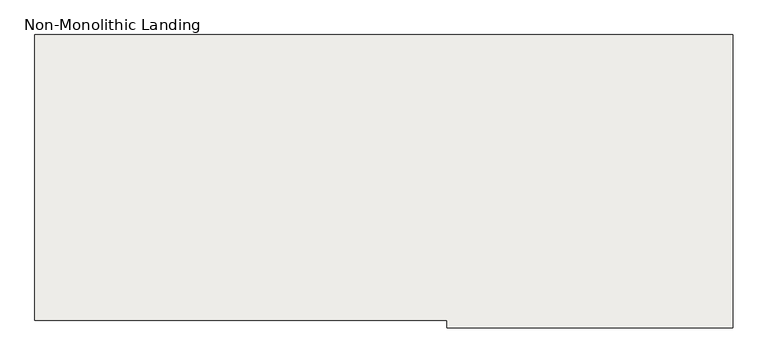
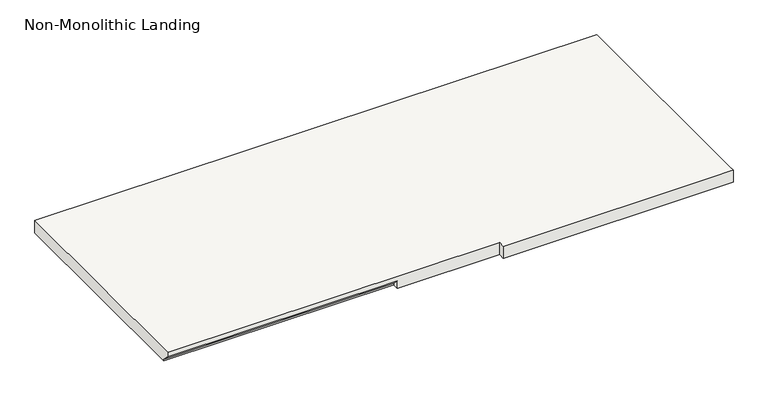
"""IFC4 building model written with IfcOpenShell, lengths in millimetres: slab geometry, Non-Monolithic Landing."""

from ifc_helpers import new_model, si_unit, origin, place, context, project, spatial, faceted_brep, source, transform, mapped, element, save


def non_monolithic_landing_1722db8f(model_context):
    return source(origin(), model_context, "Body", "Brep", [
        faceted_brep([(-3617.4415084, -19522.1851539, 27586.2339133), (-3617.4415084, -19496.7851539, 27560.8339133), (-2703.0415084, -19496.7851539, 27560.8339133), (-2703.0415084, -19522.1851539, 27586.2339133), (-2296.6415084, -19522.1851539, 27605.2839133), (-2296.6415084, -19547.5851539, 27605.2839133), (-1382.2415084, -19547.5851539, 27605.2839133), (-1382.2415084, -19522.1851539, 27605.2839133), (-1382.2415084, -18607.7851539, 27605.2839133), (-3617.4415084, -18607.7851539, 27605.2839133), (-3617.4415084, -19522.1851539, 27605.2839133), (-2703.0415084, -19496.7851539, 27554.4839133), (-3617.4415084, -19496.7851539, 27554.4839133), (-3617.4415084, -18607.7851539, 27554.4839133), (-1382.2415084, -18607.7851539, 27554.4839133), (-1382.2415084, -19522.1851539, 27554.4839133), (-1382.2415084, -19547.5851539, 27554.4839133), (-2296.6415084, -19547.5851539, 27554.4839133), (-2296.6415084, -19522.1851539, 27554.4839133), (-2703.0415084, -19522.1851539, 27554.4839133)], [[[0, 1, 2, 3]], [[4, 5, 6, 7, 8, 9, 10]], [[11, 12, 13, 14, 15, 16, 17, 18, 19]], [[12, 11, 2, 1]], [[11, 19, 3, 2]], [[4, 10, 0, 3, 19, 18]], [[5, 4, 18, 17]], [[6, 5, 17, 16]], [[7, 6, 16, 15]], [[8, 7, 15, 14]], [[9, 8, 14, 13]], [[10, 9, 13, 12, 1, 0]]]),
    ])


if __name__ == "__main__":
    model = new_model("IFC4")
    model_context = context("Model", 3, world=origin())
    ifc_project = project(units=[si_unit("LENGTHUNIT", "METRE", prefix="MILLI")], contexts=[model_context])
    site = spatial("IfcSite", under=ifc_project)
    building = spatial("IfcBuilding", under=site)
    placement = place(None, origin())
    non_monolithic_landing_shape = non_monolithic_landing_1722db8f(model_context)
    element("IfcSlab", 1, ObjectType="Non-Monolithic Landing", at=placement, inside=building, context=model_context, shape_type="MappedRepresentation", body=[
        mapped(non_monolithic_landing_shape, transform((0.0, 0.0, 0.0), x_axis=(1.0, 0.0, 0.0), y_axis=(0.0, 1.0, 0.0), z_axis=(0.0, 0.0, 1.0))),
    ])
    save(model, "model.ifc")
